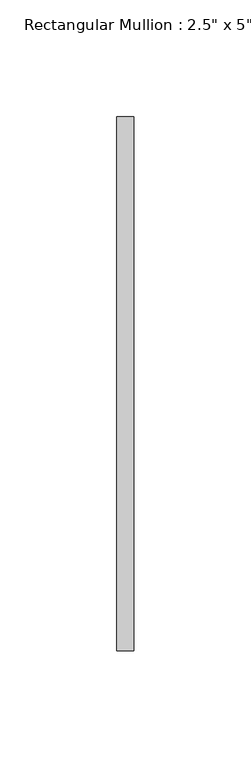
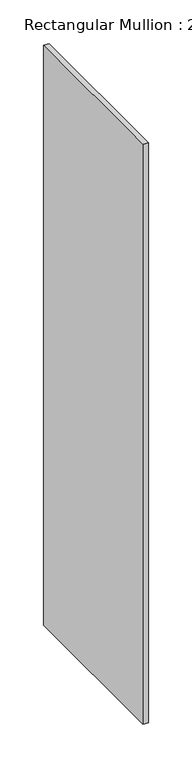
"""IFC4 building model written with IfcOpenShell, lengths in millimetres: member geometry."""

from ifc_helpers import new_model, si_unit, frame, origin, place, context, project, spatial, polyline, outline, extrude, source, transform, mapped, element, save


def member_e8dc6119(model_context):
    return source(origin(), model_context, "Body", "SweptSolid", [
        extrude(outline(polyline([(3.6195, 114.3), (3.6195, -114.3), (-3.6195, -114.3), (-3.6195, 114.3), (3.6195, 114.3)])), frame((0.0, 0.0, -812.8), z_axis=(0.0, 0.0, 1.0), x_axis=(1.0, 0.0, 0.0)), (0.0, 0.0, 1.0), 812.8),
    ])


if __name__ == "__main__":
    model = new_model("IFC4")
    model_context = context("Model", 3, world=origin())
    ifc_project = project(units=[si_unit("LENGTHUNIT", "METRE", prefix="MILLI")], contexts=[model_context])
    site = spatial("IfcSite", under=ifc_project)
    building = spatial("IfcBuilding", under=site)
    placement = place(None, origin())
    member_shape = member_e8dc6119(model_context)
    element("IfcMember", 1, ObjectType="Rectangular Mullion : 2.5\" x 5\" rectangular", at=placement, inside=building, context=model_context, shape_type="MappedRepresentation", body=[
        mapped(member_shape, transform((0.0, 0.0, 0.0), x_axis=(1.0, 0.0, 0.0), y_axis=(0.0, 1.0, 0.0), z_axis=(0.0, 0.0, 1.0))),
    ])
    save(model, "model.ifc")

# Revit data of these elements
# Type "Rectangular Mullion : 2.5\" x 5\" rectangular"
#   built-in parameter 1007304 = 0.75 (stored number, unit not read)
#   built-in parameter 1007301 = 0.011875 (stored number, unit not read)
#   built-in parameter 1007300 = 0.011875 (stored number, unit not read)
# Element 1 (IfcMember, "Rectangular Mullion : 2.5\" x 5\" rectangular")
#   Materials on its faces: "WINDOW GLASS MATERIAL"
# Materials
#   "WINDOW GLASS MATERIAL": class "Generic", colour RGB 120 120 120, transparency 0, Cost = 0
